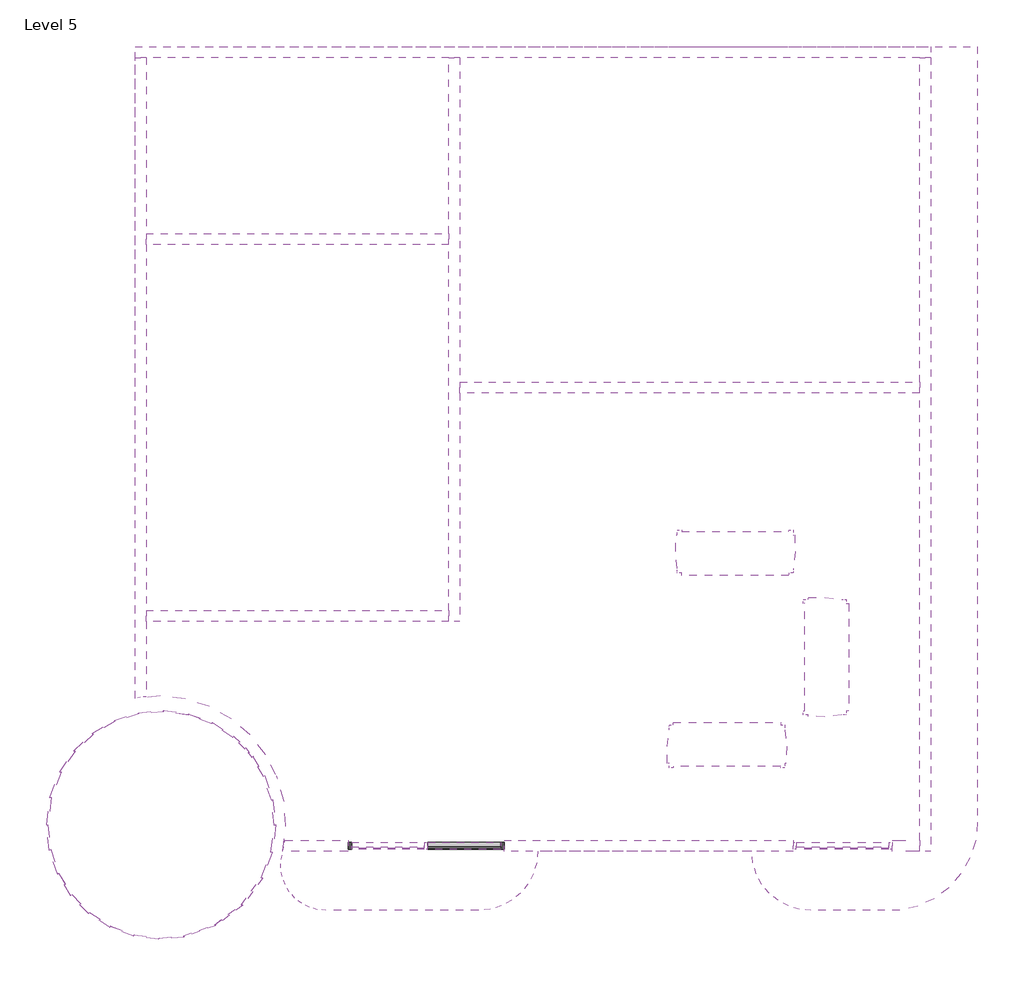
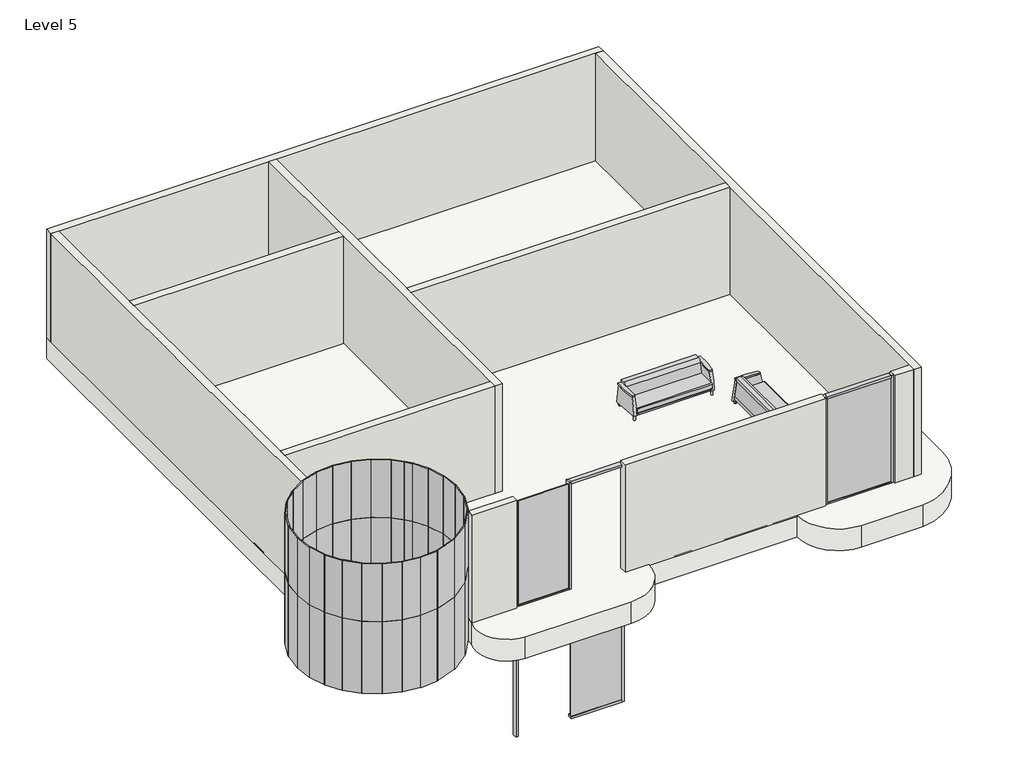
# One storey, incomplete: 59 plates, 11 members, 10 walls, 3 furniture elements, 1 slab.
"""IFC4 building model written with IfcOpenShell, lengths in millimetres."""

from ifc_helpers import new_model, si_unit, point, frame, frame_2d, origin, place, context, project, spatial, polyline, circle_curve, trimmed, segment, composite_curve, outline, extrude, faceted_brep, transform, mapped, element, save
from ifc_brep_helpers import plane_surface, revolved_surface, advanced_brep
from components import furniture_aff9b2fb, member_eaba9652, member_3f395ae9, member_0c868e12, member_7bc42366, system_panel_glazed_f1c144f9, system_panel_glazed_8ed2b2ee, system_panel_glazed_c7815b78, system_panel_glazed_220ba5f3, system_panel_glazed_11fb153e, system_panel_glazed_2f540b85, system_panel_glazed_4848e608, system_panel_glazed_8b35a0ff, system_panel_glazed_87282c25, system_panel_glazed_6d1bb68c, system_panel_glazed_cb3ffd69, system_panel_glazed_404d015f, system_panel_glazed_7b556abe, system_panel_glazed_370bf902

model = new_model("IFC4")

# Units and contexts
model_context = context("Model", 3, world=origin())
ifc_project = project(units=[si_unit("LENGTHUNIT", "METRE", prefix="MILLI")], contexts=[model_context])

# Site, building, storey
site = spatial("IfcSite", under=ifc_project)
building = spatial("IfcBuilding", under=site)
storey = spatial("IfcBuildingStorey", under=building, Name="Level 5", Elevation=12192.0)

# Furniture
placement = place(None, origin())
furniture_shape = furniture_aff9b2fb(model_context)
element("IfcFurniture", 1, ObjectType="Sofa-Pensi : 84\"", at=placement, inside=storey, context=model_context, shape_type="MappedRepresentation", body=[
    mapped(furniture_shape, transform((-2244.8524991, 3650.1964615, 14630.4), x_axis=(1.0, 0.0, 0.0), y_axis=(0.0, 1.0, 0.0), z_axis=(0.0, 0.0, 1.0))),
])
element("IfcFurniture", 2, ObjectType="Sofa-Pensi : 84\"", at=placement, inside=storey, context=model_context, shape_type="MappedRepresentation", body=[
    mapped(furniture_shape, transform((-12.736413, 1720.492712, 14630.4), x_axis=(0.0, 1.0, 0.0), y_axis=(-1.0, 0.0, 0.0), z_axis=(0.0, 0.0, 1.0))),
])
element("IfcFurniture", 3, ObjectType="Sofa-Pensi : 84\"", at=placement, inside=storey, context=model_context, shape_type="MappedRepresentation", body=[
    mapped(furniture_shape, transform((-1840.0399991, 648.4161336, 14630.4), x_axis=(-1.0, 0.0, 0.0), y_axis=(0.0, -1.0, 0.0), z_axis=(0.0, 0.0, 1.0))),
])

# Members
member_shape = member_eaba9652(model_context)
element("IfcMember", 4, ObjectType="Rectangular Mullion : 2.5\" x 5\" rectangular", at=placement, inside=storey, context=model_context, shape_type="MappedRepresentation", body=[
    mapped(member_shape, transform((-7672.5789001, -1482.8937024, 14605.0), x_axis=(-1.0, 0.0, 0.0), y_axis=(0.0, 1.0, 0.0), z_axis=(0.0, 0.0, -1.0))),
])
member_2_shape = member_3f395ae9(model_context)
element("IfcMember", 5, ObjectType="Rectangular Mullion : 2.5\" x 5\" rectangular", at=placement, inside=storey, context=model_context, shape_type="MappedRepresentation", body=[
    mapped(member_2_shape, transform((-9111.7115512, -1482.8937024, 10972.8), x_axis=(-1.0, 0.0, 0.0), y_axis=(0.0, 1.0, 0.0), z_axis=(0.0, 0.0, -1.0))),
])
element("IfcMember", 6, ObjectType="Rectangular Mullion : 2.5\" x 5\" rectangular", at=placement, inside=storey, context=model_context, shape_type="MappedRepresentation", body=[
    mapped(member_2_shape, transform((-899.4462491, -1482.8937024, 14605.0), x_axis=(-1.0, 0.0, 0.0), y_axis=(0.0, 1.0, 0.0), z_axis=(0.0, 0.0, -1.0))),
])
element("IfcMember", 7, ObjectType="Rectangular Mullion : 2.5\" x 5\" rectangular", at=placement, inside=storey, context=model_context, shape_type="MappedRepresentation", body=[
    mapped(member_2_shape, transform((-6233.4462491, -1482.8937024, 14020.8), x_axis=(1.0, 0.0, 0.0), y_axis=(0.0, 1.0, 0.0), z_axis=(0.0, 0.0, 1.0))),
])
element("IfcMember", 8, ObjectType="Rectangular Mullion : 2.5\" x 5\" rectangular", at=placement, inside=storey, context=model_context, shape_type="MappedRepresentation", body=[
    mapped(member_2_shape, transform((929.3537509, -1482.8937024, 17653.0), x_axis=(1.0, 0.0, 0.0), y_axis=(0.0, 1.0, 0.0), z_axis=(0.0, 0.0, 1.0))),
])
member_3_shape = member_0c868e12(model_context)
element("IfcMember", 9, ObjectType="Rectangular Mullion : 2.5\" x 5\" rectangular", at=placement, inside=storey, context=model_context, shape_type="MappedRepresentation", body=[
    mapped(member_3_shape, transform((-9048.2115512, -1482.8937024, 14020.8), x_axis=(0.0, 0.0, 1.0), y_axis=(0.0, 1.0, 0.0), z_axis=(-1.0, 0.0, 0.0))),
])
element("IfcMember", 10, ObjectType="Rectangular Mullion : 2.5\" x 5\" rectangular", at=placement, inside=storey, context=model_context, shape_type="MappedRepresentation", body=[
    mapped(member_3_shape, transform((-7640.8289001, -1482.8937024, 17653.0), x_axis=(0.0, 0.0, 1.0), y_axis=(0.0, 1.0, 0.0), z_axis=(-1.0, 0.0, 0.0))),
])
element("IfcMember", 11, ObjectType="Rectangular Mullion : 2.5\" x 5\" rectangular", at=placement, inside=storey, context=model_context, shape_type="MappedRepresentation", body=[
    mapped(member_3_shape, transform((-6296.9462491, -1482.8937024, 10972.8), x_axis=(0.0, 0.0, -1.0), y_axis=(0.0, 1.0, 0.0), z_axis=(1.0, 0.0, 0.0))),
])
element("IfcMember", 12, ObjectType="Rectangular Mullion : 2.5\" x 5\" rectangular", at=placement, inside=storey, context=model_context, shape_type="MappedRepresentation", body=[
    mapped(member_3_shape, transform((-7704.3289001, -1482.8937024, 14605.0), x_axis=(0.0, 0.0, -1.0), y_axis=(0.0, 1.0, 0.0), z_axis=(1.0, 0.0, 0.0))),
])
member_4_shape = member_7bc42366(model_context)
element("IfcMember", 13, ObjectType="Rectangular Mullion : 2.5\" x 5\" rectangular", at=placement, inside=storey, context=model_context, shape_type="MappedRepresentation", body=[
    mapped(member_4_shape, transform((-835.9462491, -1482.8937024, 17653.0), x_axis=(0.0, 0.0, 1.0), y_axis=(0.0, 1.0, 0.0), z_axis=(-1.0, 0.0, 0.0))),
])
element("IfcMember", 14, ObjectType="Rectangular Mullion : 2.5\" x 5\" rectangular", at=placement, inside=storey, context=model_context, shape_type="MappedRepresentation", body=[
    mapped(member_4_shape, transform((865.8537509, -1482.8937024, 14605.0), x_axis=(0.0, 0.0, -1.0), y_axis=(0.0, 1.0, 0.0), z_axis=(1.0, 0.0, 0.0))),
])

# Plates
system_panel_glazed_shape = system_panel_glazed_f1c144f9(model_context)
element("IfcPlate", 15, ObjectType="System Panel : Glazed", at=placement, inside=storey, context=model_context, shape_type="MappedRepresentation", body=[
    mapped(system_panel_glazed_shape, transform((-14541.9245022, -346.5978939, 14605.0), x_axis=(-0.3551689475306269, -0.9348021281051873, 0.0), y_axis=(0.9348021281051873, -0.3551689475306269, 0.0), z_axis=(0.0, 0.0, 1.0))),
])
element("IfcPlate", 16, ObjectType="System Panel : Glazed", at=placement, inside=storey, context=model_context, shape_type="MappedRepresentation", body=[
    mapped(system_panel_glazed_shape, transform((-10582.1178502, -1851.0877948, 14605.0), x_axis=(0.35516894753064066, 0.934802128105182, 0.0), y_axis=(-0.934802128105182, 0.35516894753064066, 0.0), z_axis=(0.0, 0.0, 1.0))),
])
element("IfcPlate", 17, ObjectType="System Panel : Glazed", at=placement, inside=storey, context=model_context, shape_type="MappedRepresentation", body=[
    mapped(system_panel_glazed_shape, transform((-10459.5232171, -1354.5613954, 14605.0), x_axis=(0.12073632210407238, 0.9926846128175765, 0.0), y_axis=(-0.9926846128175765, 0.12073632210407238, 0.0), z_axis=(0.0, 0.0, 1.0))),
])
element("IfcPlate", 18, ObjectType="System Panel : Glazed", at=placement, inside=storey, context=model_context, shape_type="MappedRepresentation", body=[
    mapped(system_panel_glazed_shape, transform((-14664.5191354, -843.1242933, 14605.0), x_axis=(-0.12073632210406239, -0.9926846128175777, 0.0), y_axis=(0.9926846128175777, -0.12073632210406239, 0.0), z_axis=(0.0, 0.0, 1.0))),
])
system_panel_glazed_2_shape = system_panel_glazed_8ed2b2ee(model_context)
element("IfcPlate", 19, ObjectType="System Panel : Glazed", at=placement, inside=storey, context=model_context, shape_type="MappedRepresentation", body=[
    mapped(system_panel_glazed_2_shape, transform((-11841.3777431, -3082.3793017, 14605.0), x_axis=(0.9398911711666007, 0.3414741371803665, 0.0), y_axis=(-0.3414741371803665, 0.9398911711666007, 0.0), z_axis=(0.0, 0.0, 1.0))),
])
element("IfcPlate", 20, ObjectType="System Panel : Glazed", at=placement, inside=storey, context=model_context, shape_type="MappedRepresentation", body=[
    mapped(system_panel_glazed_2_shape, transform((-10858.9635423, -2345.1728692, 14605.0), x_axis=(0.5905687200141164, 0.8069873524045393, 0.0), y_axis=(-0.8069873524045393, 0.5905687200141164, 0.0), z_axis=(0.0, 0.0, 1.0))),
])
element("IfcPlate", 21, ObjectType="System Panel : Glazed", at=placement, inside=storey, context=model_context, shape_type="MappedRepresentation", body=[
    mapped(system_panel_glazed_2_shape, transform((-11295.3522982, -2786.8279712, 14605.0), x_axis=(0.7998453025525061, 0.6002062078858317, 0.0), y_axis=(-0.6002062078858317, 0.7998453025525061, 0.0), z_axis=(0.0, 0.0, 1.0))),
])
system_panel_glazed_3_shape = system_panel_glazed_c7815b78(model_context)
element("IfcPlate", 22, ObjectType="System Panel : Glazed", at=placement, inside=storey, context=model_context, shape_type="MappedRepresentation", body=[
    mapped(system_panel_glazed_3_shape, transform((-10454.4737362, -864.5204039, 14605.0), x_axis=(-0.11050163420416614, 0.993875942378227, 0.0), y_axis=(-0.993875942378227, -0.11050163420416614, 0.0), z_axis=(0.0, 0.0, 1.0))),
])
element("IfcPlate", 23, ObjectType="System Panel : Glazed", at=placement, inside=storey, context=model_context, shape_type="MappedRepresentation", body=[
    mapped(system_panel_glazed_3_shape, transform((-14669.5686163, -1333.1652848, 14605.0), x_axis=(0.11050163420415136, -0.9938759423782286, 0.0), y_axis=(0.9938759423782286, 0.11050163420415136, 0.0), z_axis=(0.0, 0.0, 1.0))),
])
element("IfcPlate", 24, ObjectType="System Panel : Glazed", at=placement, inside=storey, context=model_context, shape_type="MappedRepresentation", body=[
    mapped(system_panel_glazed_3_shape, transform((-11410.1424167, 681.5611944, 14605.0), x_axis=(-0.8396018558176894, 0.5432022861766066, 0.0), y_axis=(-0.5432022861766066, -0.8396018558176894, 0.0), z_axis=(0.0, 0.0, 1.0))),
])
element("IfcPlate", 25, ObjectType="System Panel : Glazed", at=placement, inside=storey, context=model_context, shape_type="MappedRepresentation", body=[
    mapped(system_panel_glazed_3_shape, transform((-13212.0893695, 919.590846, 14605.0), x_axis=(-0.9518517343814786, -0.3065587639506839, 0.0), y_axis=(0.3065587639506839, -0.9518517343814786, 0.0), z_axis=(0.0, 0.0, 1.0))),
])
element("IfcPlate", 26, ObjectType="System Panel : Glazed", at=placement, inside=storey, context=model_context, shape_type="MappedRepresentation", body=[
    mapped(system_panel_glazed_3_shape, transform((-12839.7224363, -3201.1142893, 14605.0), x_axis=(0.9913878918151698, -0.1309581916577702, 0.0), y_axis=(0.1309581916577702, 0.9913878918151698, 0.0), z_axis=(0.0, 0.0, 1.0))),
])
element("IfcPlate", 27, ObjectType="System Panel : Glazed", at=placement, inside=storey, context=model_context, shape_type="MappedRepresentation", body=[
    mapped(system_panel_glazed_3_shape, transform((-14365.783041, -2213.7896382, 14605.0), x_axis=(0.5257859322352114, -0.8506169252157811, 0.0), y_axis=(0.8506169252157811, 0.5257859322352114, 0.0), z_axis=(0.0, 0.0, 1.0))),
])
element("IfcPlate", 28, ObjectType="System Panel : Glazed", at=placement, inside=storey, context=model_context, shape_type="MappedRepresentation", body=[
    mapped(system_panel_glazed_3_shape, transform((-13713.8999358, -2879.2468831, 14605.0), x_axis=(0.8396018558176804, -0.5432022861766203, 0.0), y_axis=(0.5432022861766203, 0.8396018558176804, 0.0), z_axis=(0.0, 0.0, 1.0))),
])
element("IfcPlate", 29, ObjectType="System Panel : Glazed", at=placement, inside=storey, context=model_context, shape_type="MappedRepresentation", body=[
    mapped(system_panel_glazed_3_shape, transform((-14014.4059364, 446.2272921, 14605.0), x_axis=(-0.7286232370002992, -0.6849147235263715, 0.0), y_axis=(0.6849147235263715, -0.7286232370002992, 0.0), z_axis=(0.0, 0.0, 1.0))),
])
element("IfcPlate", 30, ObjectType="System Panel : Glazed", at=placement, inside=storey, context=model_context, shape_type="MappedRepresentation", body=[
    mapped(system_panel_glazed_3_shape, transform((-12284.3199161, 1003.4286006, 14605.0), x_axis=(-0.9913878918151723, 0.1309581916577514, 0.0), y_axis=(-0.1309581916577514, -0.9913878918151723, 0.0), z_axis=(0.0, 0.0, 1.0))),
])
element("IfcPlate", 31, ObjectType="System Panel : Glazed", at=placement, inside=storey, context=model_context, shape_type="MappedRepresentation", body=[
    mapped(system_panel_glazed_3_shape, transform((-12752.8652893, 1013.0855973, 14605.0), x_axis=(-0.9959419324521102, -0.08999815100076568, 0.0), y_axis=(0.08999815100076568, -0.9959419324521102, 0.0), z_axis=(0.0, 0.0, 1.0))),
])
element("IfcPlate", 32, ObjectType="System Panel : Glazed", at=placement, inside=storey, context=model_context, shape_type="MappedRepresentation", body=[
    mapped(system_panel_glazed_3_shape, transform((-11829.3381514, 891.0915272, 14605.0), x_axis=(-0.9384120429483949, 0.34551821608913763, 0.0), y_axis=(-0.34551821608913763, -0.9384120429483949, 0.0), z_axis=(0.0, 0.0, 1.0))),
])
element("IfcPlate", 33, ObjectType="System Panel : Glazed", at=placement, inside=storey, context=model_context, shape_type="MappedRepresentation", body=[
    mapped(system_panel_glazed_3_shape, transform((-10557.4115054, -407.3204039, 14605.0), x_axis=(-0.32610773266043674, 0.9453326116764772, 0.0), y_axis=(-0.9453326116764772, -0.32610773266043674, 0.0), z_axis=(0.0, 0.0, 1.0))),
])
element("IfcPlate", 34, ObjectType="System Panel : Glazed", at=placement, inside=storey, context=model_context, shape_type="MappedRepresentation", body=[
    mapped(system_panel_glazed_3_shape, transform((-12371.1770631, -3210.771286, 14605.0), x_axis=(0.9959419324521115, 0.08999815100075, 0.0), y_axis=(-0.08999815100075, 0.9959419324521115, 0.0), z_axis=(0.0, 0.0, 1.0))),
])
element("IfcPlate", 35, ObjectType="System Panel : Glazed", at=placement, inside=storey, context=model_context, shape_type="MappedRepresentation", body=[
    mapped(system_panel_glazed_3_shape, transform((-13294.7042011, -3088.7772159, 14605.0), x_axis=(0.9384120429483891, -0.34551821608915334, 0.0), y_axis=(0.34551821608915334, 0.9384120429483891, 0.0), z_axis=(0.0, 0.0, 1.0))),
])
element("IfcPlate", 36, ObjectType="System Panel : Glazed", at=placement, inside=storey, context=model_context, shape_type="MappedRepresentation", body=[
    mapped(system_panel_glazed_3_shape, transform((-14076.8350959, -2582.7572647, 14605.0), x_axis=(0.6997834615185511, -0.7143550286692988, 0.0), y_axis=(0.7143550286692988, 0.6997834615185511, 0.0), z_axis=(0.0, 0.0, 1.0))),
])
element("IfcPlate", 37, ObjectType="System Panel : Glazed", at=placement, inside=storey, context=model_context, shape_type="MappedRepresentation", body=[
    mapped(system_panel_glazed_3_shape, transform((-14566.6308471, -1790.3652848, 14605.0), x_axis=(0.32610773266042153, -0.9453326116764824, 0.0), y_axis=(0.9453326116764824, 0.32610773266042153, 0.0), z_axis=(0.0, 0.0, 1.0))),
])
element("IfcPlate", 38, ObjectType="System Panel : Glazed", at=placement, inside=storey, context=model_context, shape_type="MappedRepresentation", body=[
    mapped(system_panel_glazed_3_shape, transform((-14318.3113206, 89.4787227, 14605.0), x_axis=(-0.5603879632167612, -0.8282302401396425, 0.0), y_axis=(0.8282302401396425, -0.5603879632167612, 0.0), z_axis=(0.0, 0.0, 1.0))),
])
element("IfcPlate", 39, ObjectType="System Panel : Glazed", at=placement, inside=storey, context=model_context, shape_type="MappedRepresentation", body=[
    mapped(system_panel_glazed_3_shape, transform((-13639.5625299, 727.5108588, 14605.0), x_axis=(-0.8612707706620223, -0.508146297441245, 0.0), y_axis=(0.508146297441245, -0.8612707706620223, 0.0), z_axis=(0.0, 0.0, 1.0))),
])
system_panel_glazed_4_shape = system_panel_glazed_220ba5f3(model_context)
element("IfcPlate", 40, ObjectType="System Panel : Glazed", at=placement, inside=storey, context=model_context, shape_type="MappedRepresentation", body=[
    mapped(system_panel_glazed_4_shape, transform((-10742.3305673, -4.7597883, 14605.0), x_axis=(-0.5152811917631037, 0.8570211744263939, 0.0), y_axis=(-0.8570211744263939, -0.5152811917631037, 0.0), z_axis=(0.0, 0.0, 1.0))),
])
system_panel_glazed_5_shape = system_panel_glazed_11fb153e(model_context)
element("IfcPlate", 41, ObjectType="System Panel : Glazed", at=placement, inside=storey, context=model_context, shape_type="MappedRepresentation", body=[
    mapped(system_panel_glazed_5_shape, transform((-11098.0043985, 445.2241463, 14605.0), x_axis=(-0.7256671855033587, 0.6880458821064435, 0.0), y_axis=(-0.6880458821064435, -0.7256671855033587, 0.0), z_axis=(0.0, 0.0, 1.0))),
])
system_panel_glazed_6_shape = system_panel_glazed_2f540b85(model_context)
element("IfcPlate", 42, ObjectType="System Panel : Glazed", at=placement, inside=storey, context=model_context, shape_type="MappedRepresentation", body=[
    mapped(system_panel_glazed_6_shape, transform((-10917.0903061, 255.9395759, 14605.0), x_axis=(-0.6357445726375758, 0.7718995001694626, 0.0), y_axis=(-0.7718995001694626, -0.6357445726375758, 0.0), z_axis=(0.0, 0.0, 1.0))),
])
system_panel_glazed_7_shape = system_panel_glazed_4848e608(model_context)
element("IfcPlate", 43, ObjectType="System Panel : Glazed", at=placement, inside=storey, context=model_context, shape_type="MappedRepresentation", body=[
    mapped(system_panel_glazed_7_shape, transform((-14669.5686163, -1333.1652848, 16637.0), x_axis=(0.11050163420415136, -0.9938759423782286, 0.0), y_axis=(0.9938759423782286, 0.11050163420415136, 0.0), z_axis=(0.0, 0.0, 1.0))),
])
element("IfcPlate", 44, ObjectType="System Panel : Glazed", at=placement, inside=storey, context=model_context, shape_type="MappedRepresentation", body=[
    mapped(system_panel_glazed_7_shape, transform((-14365.783041, -2213.7896382, 16637.0), x_axis=(0.5257859322352114, -0.8506169252157811, 0.0), y_axis=(0.8506169252157811, 0.5257859322352114, 0.0), z_axis=(0.0, 0.0, 1.0))),
])
element("IfcPlate", 45, ObjectType="System Panel : Glazed", at=placement, inside=storey, context=model_context, shape_type="MappedRepresentation", body=[
    mapped(system_panel_glazed_7_shape, transform((-13713.8999358, -2879.2468831, 16637.0), x_axis=(0.8396018558176805, -0.5432022861766201, 0.0), y_axis=(0.5432022861766201, 0.8396018558176805, 0.0), z_axis=(0.0, 0.0, 1.0))),
])
element("IfcPlate", 46, ObjectType="System Panel : Glazed", at=placement, inside=storey, context=model_context, shape_type="MappedRepresentation", body=[
    mapped(system_panel_glazed_7_shape, transform((-12839.7224363, -3201.1142893, 16637.0), x_axis=(0.9913878918151698, -0.13095819165777017, 0.0), y_axis=(0.13095819165777017, 0.9913878918151698, 0.0), z_axis=(0.0, 0.0, 1.0))),
])
element("IfcPlate", 47, ObjectType="System Panel : Glazed", at=placement, inside=storey, context=model_context, shape_type="MappedRepresentation", body=[
    mapped(system_panel_glazed_7_shape, transform((-12371.1770631, -3210.771286, 16637.0), x_axis=(0.9959419324521115, 0.08999815100075001, 0.0), y_axis=(-0.08999815100075001, 0.9959419324521115, 0.0), z_axis=(0.0, 0.0, 1.0))),
])
element("IfcPlate", 48, ObjectType="System Panel : Glazed", at=placement, inside=storey, context=model_context, shape_type="MappedRepresentation", body=[
    mapped(system_panel_glazed_7_shape, transform((-13294.7042011, -3088.7772159, 16637.0), x_axis=(0.9384120429483891, -0.34551821608915334, 0.0), y_axis=(0.34551821608915334, 0.9384120429483891, 0.0), z_axis=(0.0, 0.0, 1.0))),
])
element("IfcPlate", 49, ObjectType="System Panel : Glazed", at=placement, inside=storey, context=model_context, shape_type="MappedRepresentation", body=[
    mapped(system_panel_glazed_7_shape, transform((-14076.8350959, -2582.7572647, 16637.0), x_axis=(0.6997834615185511, -0.7143550286692988, 0.0), y_axis=(0.7143550286692988, 0.6997834615185511, 0.0), z_axis=(0.0, 0.0, 1.0))),
])
element("IfcPlate", 50, ObjectType="System Panel : Glazed", at=placement, inside=storey, context=model_context, shape_type="MappedRepresentation", body=[
    mapped(system_panel_glazed_7_shape, transform((-14566.6308471, -1790.3652848, 16637.0), x_axis=(0.3261077326604215, -0.9453326116764824, 0.0), y_axis=(0.9453326116764824, 0.3261077326604215, 0.0), z_axis=(0.0, 0.0, 1.0))),
])
element("IfcPlate", 51, ObjectType="System Panel : Glazed", at=placement, inside=storey, context=model_context, shape_type="MappedRepresentation", body=[
    mapped(system_panel_glazed_7_shape, transform((-10454.4737362, -864.5204039, 16637.0), x_axis=(-0.11050163420416613, 0.993875942378227, 0.0), y_axis=(-0.993875942378227, -0.11050163420416613, 0.0), z_axis=(0.0, 0.0, 1.0))),
])
element("IfcPlate", 52, ObjectType="System Panel : Glazed", at=placement, inside=storey, context=model_context, shape_type="MappedRepresentation", body=[
    mapped(system_panel_glazed_7_shape, transform((-10557.4115054, -407.3204039, 16637.0), x_axis=(-0.32610773266043674, 0.9453326116764772, 0.0), y_axis=(-0.9453326116764772, -0.32610773266043674, 0.0), z_axis=(0.0, 0.0, 1.0))),
])
element("IfcPlate", 53, ObjectType="System Panel : Glazed", at=placement, inside=storey, context=model_context, shape_type="MappedRepresentation", body=[
    mapped(system_panel_glazed_7_shape, transform((-11410.1424167, 681.5611944, 16637.0), x_axis=(-0.8396018558176894, 0.5432022861766066, 0.0), y_axis=(-0.5432022861766066, -0.8396018558176894, 0.0), z_axis=(0.0, 0.0, 1.0))),
])
element("IfcPlate", 54, ObjectType="System Panel : Glazed", at=placement, inside=storey, context=model_context, shape_type="MappedRepresentation", body=[
    mapped(system_panel_glazed_7_shape, transform((-11829.3381514, 891.0915272, 16637.0), x_axis=(-0.9384120429483949, 0.3455182160891376, 0.0), y_axis=(-0.3455182160891376, -0.9384120429483949, 0.0), z_axis=(0.0, 0.0, 1.0))),
])
element("IfcPlate", 55, ObjectType="System Panel : Glazed", at=placement, inside=storey, context=model_context, shape_type="MappedRepresentation", body=[
    mapped(system_panel_glazed_7_shape, transform((-12284.3199161, 1003.4286006, 16637.0), x_axis=(-0.9913878918151723, 0.13095819165775144, 0.0), y_axis=(-0.13095819165775144, -0.9913878918151723, 0.0), z_axis=(0.0, 0.0, 1.0))),
])
element("IfcPlate", 56, ObjectType="System Panel : Glazed", at=placement, inside=storey, context=model_context, shape_type="MappedRepresentation", body=[
    mapped(system_panel_glazed_7_shape, transform((-12752.8652893, 1013.0855973, 16637.0), x_axis=(-0.9959419324521102, -0.08999815100076569, 0.0), y_axis=(0.08999815100076569, -0.9959419324521102, 0.0), z_axis=(0.0, 0.0, 1.0))),
])
element("IfcPlate", 57, ObjectType="System Panel : Glazed", at=placement, inside=storey, context=model_context, shape_type="MappedRepresentation", body=[
    mapped(system_panel_glazed_7_shape, transform((-13212.0893695, 919.590846, 16637.0), x_axis=(-0.9518517343814786, -0.3065587639506839, 0.0), y_axis=(0.3065587639506839, -0.9518517343814786, 0.0), z_axis=(0.0, 0.0, 1.0))),
])
element("IfcPlate", 58, ObjectType="System Panel : Glazed", at=placement, inside=storey, context=model_context, shape_type="MappedRepresentation", body=[
    mapped(system_panel_glazed_7_shape, transform((-13639.5625299, 727.5108588, 16637.0), x_axis=(-0.8612707706620224, -0.5081462974412448, 0.0), y_axis=(0.5081462974412448, -0.8612707706620224, 0.0), z_axis=(0.0, 0.0, 1.0))),
])
element("IfcPlate", 59, ObjectType="System Panel : Glazed", at=placement, inside=storey, context=model_context, shape_type="MappedRepresentation", body=[
    mapped(system_panel_glazed_7_shape, transform((-14014.4059364, 446.2272921, 16637.0), x_axis=(-0.7286232370002992, -0.6849147235263715, 0.0), y_axis=(0.6849147235263715, -0.7286232370002992, 0.0), z_axis=(0.0, 0.0, 1.0))),
])
element("IfcPlate", 60, ObjectType="System Panel : Glazed", at=placement, inside=storey, context=model_context, shape_type="MappedRepresentation", body=[
    mapped(system_panel_glazed_7_shape, transform((-14318.3113206, 89.4787227, 16637.0), x_axis=(-0.5603879632167612, -0.8282302401396425, 0.0), y_axis=(0.8282302401396425, -0.5603879632167612, 0.0), z_axis=(0.0, 0.0, 1.0))),
])
system_panel_glazed_8_shape = system_panel_glazed_8b35a0ff(model_context)
element("IfcPlate", 61, ObjectType="System Panel : Glazed", at=placement, inside=storey, context=model_context, shape_type="MappedRepresentation", body=[
    mapped(system_panel_glazed_8_shape, transform((-10742.3305673, -4.7597883, 16637.0), x_axis=(-0.5152811917631037, 0.8570211744263939, 0.0), y_axis=(-0.8570211744263939, -0.5152811917631037, 0.0), z_axis=(0.0, 0.0, 1.0))),
])
system_panel_glazed_9_shape = system_panel_glazed_87282c25(model_context)
element("IfcPlate", 62, ObjectType="System Panel : Glazed", at=placement, inside=storey, context=model_context, shape_type="MappedRepresentation", body=[
    mapped(system_panel_glazed_9_shape, transform((-10917.0903061, 255.9395759, 16637.0), x_axis=(-0.6357445726375756, 0.7718995001694628, 0.0), y_axis=(-0.7718995001694628, -0.6357445726375756, 0.0), z_axis=(0.0, 0.0, 1.0))),
])
system_panel_glazed_10_shape = system_panel_glazed_6d1bb68c(model_context)
element("IfcPlate", 63, ObjectType="System Panel : Glazed", at=placement, inside=storey, context=model_context, shape_type="MappedRepresentation", body=[
    mapped(system_panel_glazed_10_shape, transform((-11098.0043985, 445.2241463, 16637.0), x_axis=(-0.7256671855033587, 0.6880458821064435, 0.0), y_axis=(-0.6880458821064435, -0.7256671855033587, 0.0), z_axis=(0.0, 0.0, 1.0))),
])
system_panel_glazed_11_shape = system_panel_glazed_cb3ffd69(model_context)
element("IfcPlate", 64, ObjectType="System Panel : Glazed", at=placement, inside=storey, context=model_context, shape_type="MappedRepresentation", body=[
    mapped(system_panel_glazed_11_shape, transform((-10582.1178502, -1851.0877948, 16637.0), x_axis=(0.35516894753064066, 0.934802128105182, 0.0), y_axis=(-0.934802128105182, 0.35516894753064066, 0.0), z_axis=(0.0, 0.0, 1.0))),
])
element("IfcPlate", 65, ObjectType="System Panel : Glazed", at=placement, inside=storey, context=model_context, shape_type="MappedRepresentation", body=[
    mapped(system_panel_glazed_11_shape, transform((-10459.5232171, -1354.5613954, 16637.0), x_axis=(0.12073632210407237, 0.9926846128175765, 0.0), y_axis=(-0.9926846128175765, 0.12073632210407237, 0.0), z_axis=(0.0, 0.0, 1.0))),
])
element("IfcPlate", 66, ObjectType="System Panel : Glazed", at=placement, inside=storey, context=model_context, shape_type="MappedRepresentation", body=[
    mapped(system_panel_glazed_11_shape, transform((-14541.9245022, -346.5978939, 16637.0), x_axis=(-0.3551689475306269, -0.9348021281051873, 0.0), y_axis=(0.9348021281051873, -0.3551689475306269, 0.0), z_axis=(0.0, 0.0, 1.0))),
])
element("IfcPlate", 67, ObjectType="System Panel : Glazed", at=placement, inside=storey, context=model_context, shape_type="MappedRepresentation", body=[
    mapped(system_panel_glazed_11_shape, transform((-14664.5191354, -843.1242933, 16637.0), x_axis=(-0.1207363221040624, -0.9926846128175777, 0.0), y_axis=(0.9926846128175777, -0.1207363221040624, 0.0), z_axis=(0.0, 0.0, 1.0))),
])
system_panel_glazed_12_shape = system_panel_glazed_404d015f(model_context)
element("IfcPlate", 68, ObjectType="System Panel : Glazed", at=placement, inside=storey, context=model_context, shape_type="MappedRepresentation", body=[
    mapped(system_panel_glazed_12_shape, transform((-11841.3777431, -3082.3793017, 16637.0), x_axis=(0.9398911711666007, 0.3414741371803665, 0.0), y_axis=(-0.3414741371803665, 0.9398911711666007, 0.0), z_axis=(0.0, 0.0, 1.0))),
])
element("IfcPlate", 69, ObjectType="System Panel : Glazed", at=placement, inside=storey, context=model_context, shape_type="MappedRepresentation", body=[
    mapped(system_panel_glazed_12_shape, transform((-10858.9635423, -2345.1728692, 16637.0), x_axis=(0.5905687200141163, 0.8069873524045394, 0.0), y_axis=(-0.8069873524045394, 0.5905687200141163, 0.0), z_axis=(0.0, 0.0, 1.0))),
])
element("IfcPlate", 70, ObjectType="System Panel : Glazed", at=placement, inside=storey, context=model_context, shape_type="MappedRepresentation", body=[
    mapped(system_panel_glazed_12_shape, transform((-11295.3522982, -2786.8279712, 16637.0), x_axis=(0.7998453025525061, 0.6002062078858317, 0.0), y_axis=(-0.6002062078858317, 0.7998453025525061, 0.0), z_axis=(0.0, 0.0, 1.0))),
])
system_panel_glazed_13_shape = system_panel_glazed_7b556abe(model_context)
element("IfcPlate", 71, ObjectType="System Panel : Glazed", at=placement, inside=storey, context=model_context, shape_type="MappedRepresentation", body=[
    mapped(system_panel_glazed_13_shape, transform((-6968.8875746, -1482.8937024, 11036.3), x_axis=(-1.0, 0.0, 0.0), y_axis=(0.0, -1.0, 0.0), z_axis=(0.0, 0.0, 1.0))),
])
element("IfcPlate", 72, ObjectType="System Panel : Glazed", at=placement, inside=storey, context=model_context, shape_type="MappedRepresentation", body=[
    mapped(system_panel_glazed_13_shape, transform((-8376.2702257, -1482.8937024, 14668.5), x_axis=(-1.0, 0.0, 0.0), y_axis=(0.0, -1.0, 0.0), z_axis=(0.0, 0.0, 1.0))),
])
system_panel_glazed_14_shape = system_panel_glazed_370bf902(model_context)
element("IfcPlate", 73, ObjectType="System Panel : Glazed", at=placement, inside=storey, context=model_context, shape_type="MappedRepresentation", body=[
    mapped(system_panel_glazed_14_shape, transform((14.9537509, -1482.8937024, 14668.5), x_axis=(-1.0, 0.0, 0.0), y_axis=(0.0, -1.0, 0.0), z_axis=(0.0, 0.0, 1.0))),
])

# Slab
element("IfcSlab", 74, ObjectType="Generic - 2'", at=placement, inside=storey, context=model_context, shape_type="SweptSolid", body=[
    extrude(outline(composite_curve([segment(polyline([(2504.1537509, 13274.5062976), (2504.1537509, -1051.0937024)]), True, "CONTINUOUS"), segment(trimmed(circle_curve(frame_2d((865.9099456, -1051.0937024)), 1638.2438053), [point((2504.1537509, -1051.0937024))], [point((1069.0537509, -2676.6937024))], False, "CARTESIAN"), True, "CONTINUOUS"), segment(polyline([(1069.0537509, -2676.6937024), (-569.2462491, -2676.6937024)]), True, "CONTINUOUS"), segment(trimmed(circle_curve(frame_2d((-569.2462491, -1584.4937024)), 1092.2), [point((-569.2462491, -2676.6937024))], [point((-1661.4462491, -1584.4937024))], False, "CARTESIAN"), True, "CONTINUOUS"), segment(polyline([(-1661.4462491, -1584.4937024), (-5609.8647377, -1584.4937024)]), True, "CONTINUOUS"), segment(trimmed(circle_curve(frame_2d((-6702.0647377, -1584.4937024)), 1092.2), [point((-5609.8647377, -1584.4937024))], [point((-6702.0647377, -2676.6937024))], False, "CARTESIAN"), True, "CONTINUOUS"), segment(polyline([(-6702.0647377, -2676.6937024), (-9521.4647377, -2676.6937024)]), True, "CONTINUOUS"), segment(trimmed(circle_curve(frame_2d((-9521.4647377, -1843.8920375)), 832.801665), [point((-9521.4647377, -2676.6937024))], [point((-10312.8376694, -1584.4937024))], False, "CARTESIAN"), True, "CONTINUOUS"), segment(trimmed(circle_curve(frame_2d((-12612.6150686, -1075.1054509)), 2355.5153315), [point((-10312.8376694, -1584.4937024))], [point((-13040.6462491, 1241.1937063))], True, "CARTESIAN"), True, "CONTINUOUS"), segment(polyline([(-13040.6462491, 1241.1937063), (-13040.6462491, 13274.5062976), (2504.1537509, 13274.5062976)]), True, "CONTINUOUS")], self_intersect=False)), frame((0.0, 0.0, 14020.8), z_axis=(0.0, 0.0, 1.0), x_axis=(1.0, 0.0, 0.0)), (0.0, 0.0, 1.0), 609.6),
])

# Walls
element("IfcWall", 75, ObjectType="Generic - 8\"", at=placement, inside=storey, context=model_context, shape_type="Brep", body=[
    faceted_brep([(-13040.6462491, 13071.3062976, 14605.0), (-12837.4462491, 13071.3062976, 14605.0), (-7249.4462491, 13071.3062976, 14605.0), (-7046.2462491, 13071.3062976, 14605.0), (1437.3537509, 13071.3062976, 14605.0), (1640.5537509, 13071.3062976, 14605.0), (1640.5537509, 13071.3062976, 17653.0), (1437.3537509, 13071.3062976, 17653.0), (-7046.2462491, 13071.3062976, 17653.0), (-7249.4462491, 13071.3062976, 17653.0), (-12837.4462491, 13071.3062976, 17653.0), (-13040.6462491, 13071.3062976, 17653.0), (-13040.6462491, 13274.5062976, 14605.0), (-13040.6462491, 13274.5062976, 17653.0), (1640.5537509, 13274.5062976, 17653.0), (1640.5537509, 13274.5062976, 14605.0)], [[[0, 1, 2, 3, 4, 5, 6, 7, 8, 9, 10, 11]], [[12, 13, 14, 15]], [[5, 4, 3, 2, 1, 0, 12, 15]], [[11, 10, 9, 8, 7, 6, 14, 13]], [[6, 5, 15, 14]], [[0, 11, 13, 12]]]),
])
element("IfcWall", 76, ObjectType="Generic - 8\"", at=placement, inside=storey, context=model_context, shape_type="Brep", body=[
    faceted_brep([(1437.3537509, 13071.3062976, 14605.0), (1437.3537509, 7076.9062976, 14605.0), (1437.3537509, 6873.7062976, 14605.0), (1437.3537509, -1381.2937024, 14605.0), (1437.3537509, -1584.4937024, 14605.0), (1437.3537509, -1584.4937024, 17653.0), (1437.3537509, -1381.2937024, 17653.0), (1437.3537509, 6873.7062976, 17653.0), (1437.3537509, 7076.9062976, 17653.0), (1437.3537509, 13071.3062976, 17653.0), (1640.5537509, 13071.3062976, 14605.0), (1640.5537509, 13071.3062976, 17653.0), (1640.5537509, -1584.4937024, 17653.0), (1640.5537509, -1584.4937024, 14605.0)], [[[0, 1, 2, 3, 4, 5, 6, 7, 8, 9]], [[10, 11, 12, 13]], [[4, 3, 2, 1, 0, 10, 13]], [[9, 8, 7, 6, 5, 12, 11]], [[0, 9, 11, 10]], [[5, 4, 13, 12]]]),
])
element("IfcWall", 77, ObjectType="Generic - 8\"", at=placement, inside=storey, context=model_context, shape_type="AdvancedBrep", body=[
    advanced_brep(
    [(-13040.6462491, 13071.3062976, 14605.0), (-13040.6462491, 1241.1937063, 14605.0), (-13040.6462491, 1241.1937063, 17653.0), (-13040.6462491, 13071.3062976, 17653.0), (-12837.4462491, 13071.3062976, 14605.0), (-12837.4462491, 13071.3062976, 17653.0), (-12837.4462491, 9820.1062976, 17653.0), (-12837.4462491, 9616.9062976, 17653.0), (-12837.4462491, 2862.698962, 17653.0), (-12837.4462491, 2659.498962, 17653.0), (-12837.4462491, 1269.6553935, 17653.0), (-12837.4462491, 1269.6553935, 14605.0), (-12837.4462491, 2659.498962, 14605.0), (-12837.4462491, 2862.698962, 14605.0), (-12837.4462491, 9616.9062976, 14605.0), (-12837.4462491, 9820.1062976, 14605.0)],
    [
        (0, 1),
        (1, 2),
        (2, 3),
        (3, 0),
        (4, 5),
        (5, 6),
        (6, 7),
        (7, 8),
        (8, 9),
        (9, 10),
        (10, 11),
        (11, 12),
        (12, 13),
        (13, 14),
        (14, 15),
        (15, 4),
        (0, 4),
        (11, 1, circle_curve(frame((-12612.6150686, -1075.1054509, 14605.0), z_axis=(0.0, 0.0, 1.0), x_axis=(1.0, 0.0, 0.0)), 2355.5153315)),
        (2, 10, circle_curve(frame((-12612.6150686, -1075.1054509, 17653.0), z_axis=(0.0, 0.0, -1.0), x_axis=(1.0, 0.0, 0.0)), 2355.5153315)),
        (5, 3),
    ],
    [
        plane_surface(frame((-13040.6462491, 16068.5062976, 14605.0), z_axis=(-1.0, 0.0, 0.0), x_axis=(0.0, -1.0, 0.0))),
        plane_surface(frame((-12837.4462491, 16068.5062976, 14605.0), z_axis=(1.0, 0.0, 0.0), x_axis=(0.0, 1.0, 0.0))),
        plane_surface(frame((-13040.6462491, 13172.9062976, 14605.0), z_axis=(0.0, 0.0, -1.0), x_axis=(1.0, 0.0, 0.0))),
        plane_surface(frame((-13040.6462491, 1155.046339, 17653.0), z_axis=(0.0, 0.0, 1.0), x_axis=(1.0, 0.0, 0.0))),
        plane_surface(frame((-16139.4462491, 13071.3062976, 14605.0), z_axis=(0.0, 1.0, 0.0), x_axis=(1.0, 0.0, 0.0))),
        revolved_surface(polyline([(-10257.099737100001, -1075.1054509, 17653.0), (-10257.099737100001, -1075.1054509, 14605.0)]), (-12612.6150686, -1075.1054509, 14605.0), (0.0, 0.0, 1.0)),
    ],
    [
        (0, [[1, 2, 3, 4]]),
        (1, [[5, 6, 7, 8, 9, 10, 11, 12, 13, 14, 15, 16]]),
        (2, [[-1, 17, -16, -15, -14, -13, -12, 18]]),
        (3, [[-3, 19, -10, -9, -8, -7, -6, 20]]),
        (4, [[-4, -20, -5, -17]]),
        (5, [[-2, -18, -11, -19]]),
    ],
),
])
element("IfcWall", 78, ObjectType="Generic - 8\"", at=placement, inside=storey, context=model_context, shape_type="Brep", body=[
    faceted_brep([(-7249.4462491, 13071.3062976, 14605.0), (-7249.4462491, 9820.1062976, 14605.0), (-7249.4462491, 9616.9062976, 14605.0), (-7249.4462491, 2862.698962, 14605.0), (-7249.4462491, 2659.498962, 14605.0), (-7249.4462491, 2659.498962, 17653.0), (-7249.4462491, 2862.698962, 17653.0), (-7249.4462491, 9616.9062976, 17653.0), (-7249.4462491, 9820.1062976, 17653.0), (-7249.4462491, 13071.3062976, 17653.0), (-7046.2462491, 13071.3062976, 14605.0), (-7046.2462491, 13071.3062976, 17653.0), (-7046.2462491, 7076.9062976, 17653.0), (-7046.2462491, 6873.7062976, 17653.0), (-7046.2462491, 2659.498962, 17653.0), (-7046.2462491, 2659.498962, 14605.0), (-7046.2462491, 6873.7062976, 14605.0), (-7046.2462491, 7076.9062976, 14605.0)], [[[0, 1, 2, 3, 4, 5, 6, 7, 8, 9]], [[10, 11, 12, 13, 14, 15, 16, 17]], [[4, 3, 2, 1, 0, 10, 17, 16, 15]], [[9, 8, 7, 6, 5, 14, 13, 12, 11]], [[0, 9, 11, 10]], [[5, 4, 15, 14]]]),
])
element("IfcWall", 79, ObjectType="Generic - 8\"", at=placement, inside=storey, context=model_context, shape_type="SweptSolid", body=[
    extrude(outline(polyline([(1437.3537509, 6873.7062976), (-7046.2462491, 6873.7062976), (-7046.2462491, 7076.9062976), (1437.3537509, 7076.9062976), (1437.3537509, 6873.7062976)])), frame((0.0, 0.0, 14605.0), z_axis=(0.0, 0.0, 1.0), x_axis=(1.0, 0.0, 0.0)), (0.0, 0.0, 1.0), 3048.0),
])
element("IfcWall", 80, ObjectType="Generic - 8\"", at=placement, inside=storey, context=model_context, shape_type="SweptSolid", body=[
    extrude(outline(polyline([(-12837.4462491, 9820.1062976), (-7249.4462491, 9820.1062976), (-7249.4462491, 9616.9062976), (-12837.4462491, 9616.9062976), (-12837.4462491, 9820.1062976)])), frame((0.0, 0.0, 14605.0), z_axis=(0.0, 0.0, 1.0), x_axis=(1.0, 0.0, 0.0)), (0.0, 0.0, 1.0), 3048.0),
])
element("IfcWall", 81, ObjectType="Generic - 8\"", at=placement, inside=storey, context=model_context, shape_type="SweptSolid", body=[
    extrude(outline(polyline([(-12837.4462491, 2862.698962), (-7249.4462491, 2862.698962), (-7249.4462491, 2659.498962), (-12837.4462491, 2659.498962), (-12837.4462491, 2862.698962)])), frame((0.0, 0.0, 14605.0), z_axis=(0.0, 0.0, 1.0), x_axis=(1.0, 0.0, 0.0)), (0.0, 0.0, 1.0), 3048.0),
])
element("IfcWall", 82, ObjectType="Generic - 8\"", at=placement, inside=storey, context=model_context, shape_type="SweptSolid", body=[
    extrude(outline(composite_curve([segment(polyline([(-9111.7115512, -1584.4937024), (-10312.8376694, -1584.4937024)]), True, "CONTINUOUS"), segment(trimmed(circle_curve(frame_2d((-12612.6150686, -1075.1054509)), 2355.5153315), [point((-10312.8376694, -1584.4937024))], [point((-10277.0848865, -1381.2937024))], True, "CARTESIAN"), True, "CONTINUOUS"), segment(polyline([(-10277.0848865, -1381.2937024), (-9111.7115512, -1381.2937024), (-9111.7115512, -1584.4937024)]), True, "CONTINUOUS")], self_intersect=False)), frame((0.0, 0.0, 14605.0), z_axis=(0.0, 0.0, 1.0), x_axis=(1.0, 0.0, 0.0)), (0.0, 0.0, 1.0), 3048.0),
])
element("IfcWall", 83, ObjectType="Generic - 8\"", at=placement, inside=storey, context=model_context, shape_type="SweptSolid", body=[
    extrude(outline(polyline([(-899.4462491, -1584.4937024), (-6233.4462491, -1584.4937024), (-6233.4462491, -1381.2937024), (-899.4462491, -1381.2937024), (-899.4462491, -1584.4937024)])), frame((0.0, 0.0, 14605.0), z_axis=(0.0, 0.0, 1.0), x_axis=(1.0, 0.0, 0.0)), (0.0, 0.0, 1.0), 3048.0),
])
element("IfcWall", 84, ObjectType="Generic - 8\"", at=placement, inside=storey, context=model_context, shape_type="SweptSolid", body=[
    extrude(outline(polyline([(929.3537509, -1381.2937024), (1437.3537509, -1381.2937024), (1437.3537509, -1584.4937024), (929.3537509, -1584.4937024), (929.3537509, -1381.2937024)])), frame((0.0, 0.0, 14605.0), z_axis=(0.0, 0.0, 1.0), x_axis=(1.0, 0.0, 0.0)), (0.0, 0.0, 1.0), 3048.0),
])

save(model, "model.ifc")

# Revit data of these elements
# Type "Sofa-Pensi : 84\""
#   Assembly Code = "E2020200"
#   Length = 7' - 0"
#   Frame Material = Cherry
#   Seat Material = Linen, Beige
#   Feet Material = Steel, Chrome Plated
#   Default Elevation = 0
# Type "Rectangular Mullion : 2.5\" x 5\" rectangular"
#   built-in parameter 1007304 = 0.416667 (stored number, unit not read)
#   built-in parameter 1007301 = 0.104167 (stored number, unit not read)
#   built-in parameter 1007300 = 0.104167 (stored number, unit not read)
# Type "System Panel : Glazed"
#   Construction Type Id = "GSP4R"
#   Analytic Construction = "1/8 in Pilkington single glazing"
#   Visual Light Transmittance = 0.9
#   Solar Heat Gain Coefficient = 0.86
#   Heat Transfer Coefficient (U) = 1.18115 BTU/(h·ft²·°F)
# Type "Generic - 2'"
#   Assembly Code = "B1010"
#   Function = 0
#   Layers, outside or top first: 2' - 0" no material (function 1)
# Type "Generic - 8\""
#   Assembly Code = "B2010"
#   Layers, outside or top first: 0' - 8" no material (function 1)
# Elements 1, 2, 3 (IfcFurniture, "Sofa-Pensi : 84\"")
#   Phase Created = New Construction
#   Materials on its faces: "Cherry", "Linen, Beige", "Steel, Chrome Plated"
# Elements 4, 5, 6, 7, 8, 9, 10, 11, 12, 13, 14 (IfcMember, "Rectangular Mullion : 2.5\" x 5\" rectangular")
#   Phase Created = New Construction
#   Materials on its faces: "Iron, Ductile"
# Elements 15, 16, 17, 18, 19, 20, 21, 22, 23, 24, 25, 26, 27, 28, 29, 30, 31, 32, 33, 34, 35, 36, 37, 38, 39, 40, 41, 42, 43, 44, 45, 46, 47, 48, 49, 50, 51, 52, 53, 54, 55, 56, 57, 58, 59, 60, 61, 62, 63, 64, 65, 66, 67, 68, 69, 70, 71, 72, 73 (IfcPlate, "System Panel : Glazed")
#   Phase Created = New Construction
#   Materials on its faces: "Glass"
# Element 74 (IfcSlab, "Generic - 2'")
#   Height Offset From Level = 8' - 0"
#   Phase Created = New Construction
#   Materials on its faces: "Default Floor"
# Elements 75, 76, 77, 78, 79, 80, 81, 82, 83, 84 (IfcWall, "Generic - 8\"")
#   built-in parameter 1001111 = 7' - 11"
#   Top Offset = 0' - 0"
#   Base Offset = 7' - 11"
#   Unconnected Height = 10' - 0"
#   wall height = 10' - 0"
#   Phase Created = New Construction
#   Base Constraint = Level 5
#   Materials on its faces: "Default Wall"
# Materials
#   "Cherry": class "Wood", colour RGB 226 177 128, transparency 0, Description = "Prunus Serotina", Cost = 0
#   "Linen, Beige": class "Textile", colour RGB 249 239 230, transparency 0, Description = "Linen, beige", Cost = 0
#   "Steel, Chrome Plated": class "Metal", colour RGB 17 17 17, transparency 0, Description = "Chromiuim plated steel", Cost = 0
#   "Iron, Ductile": class "Metal", colour RGB 0 0 0, transparency 0, Description = "Ductile cast iron", Cost = 0
#   "Glass": class "Glass", colour RGB 0 128 192, transparency 0.75, Description = "Soda Lime Glass", Cost = 0
#   "Default Floor": colour RGB 128 128 128, transparency 0
#   "Default Wall": colour RGB 128 128 128, transparency 0
